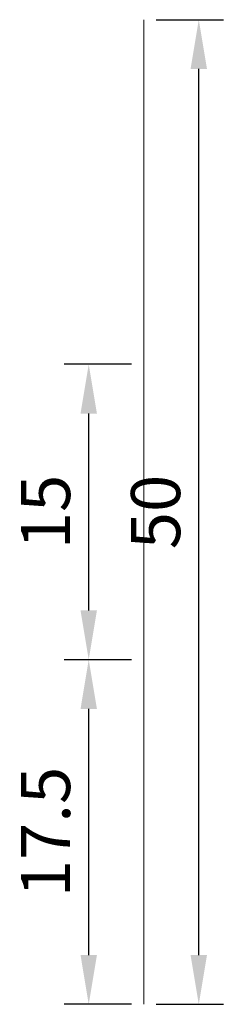
# Model space of a CAD drawing. Units: millimetres. Extents: x -6 to 912, y -42 to 105.
# Tile 1 of 2: x -6 to 4, y 55 to 105. Entities that reach past the tile are written whole.
import ezdxf

# ---------------------------------------------------------------- set-up
doc = ezdxf.new("R2010")
doc.units = ezdxf.units.MM
doc.layers.add('M-CONS', color=8, linetype='Continuous', lineweight=18)
doc.layers.add('M-DIMS', color=2, linetype='Continuous', lineweight=18)
doc.dimstyles.new('ISO-25', dxfattribs={"dimtxt": 2.5, "dimasz": 2.5, "dimexe": 1.25, "dimexo": 0.625, "dimtad": 1, "dimtxsty": 'Standard', "dimcen": 2.5, "dimadec": 0, "dimazin": 0, "dimtfac": 1, "dimtmove": 0, "dimatfit": 3, "dimfxl": 1, "dimarcsym": 0})

# ---------------------------------------------------------------- blocks, each defined once
blk = doc.blocks.new('*D8')
at = {"layer": 'Defpoints', "color": 0, "transparency": 16777216}
for p in [(0, 105.147), (2.8, 105.147), (0, 55.147)]:
    blk.add_point(p, dxfattribs=at)
at = {"layer": 'M-DIMS', "color": 0, "lineweight": -2, "transparency": 16777216}
for p, q in [((0.625, 105.147), (4.05, 105.147)), ((2.8, 57.647), (2.8, 102.647)), ((0.625, 55.147), (4.05, 55.147))]:
    blk.add_line(p, q, dxfattribs=at)
at = {"layer": 'M-DIMS', "color": 0, "transparency": 16777216}
for points in [[(2.383, 102.647), (3.217, 102.647), (2.8, 105.147)], [(2.383, 57.647), (3.217, 57.647), (2.8, 55.147)]]:
    blk.add_solid(points, dxfattribs=at)
at = {"layer": 'M-DIMS', "color": 0, "transparency": 16777216, "insert": (0.925, 80.147), "char_height": 2.5, "attachment_point": 5, "rotation": 90}
blk.add_mtext('50', dxfattribs=at)
blk = doc.blocks.new('*D9')
at = {"layer": 'Defpoints', "color": 0, "transparency": 16777216}
for p in [(-2.8, 72.647), (0, 72.647), (0, 55.147)]:
    blk.add_point(p, dxfattribs=at)
at = {"layer": 'M-DIMS', "color": 0, "lineweight": -2, "transparency": 16777216}
for p, q in [((-0.625, 72.647), (-4.05, 72.647)), ((-2.8, 57.647), (-2.8, 70.147)), ((-0.625, 55.147), (-4.05, 55.147))]:
    blk.add_line(p, q, dxfattribs=at)
at = {"layer": 'M-DIMS', "color": 0, "transparency": 16777216}
for points in [[(-3.217, 70.147), (-2.383, 70.147), (-2.8, 72.647)], [(-3.217, 57.647), (-2.383, 57.647), (-2.8, 55.147)]]:
    blk.add_solid(points, dxfattribs=at)
at = {"layer": 'M-DIMS', "color": 0, "transparency": 16777216, "insert": (-4.675, 63.897), "char_height": 2.5, "attachment_point": 5, "rotation": 90}
blk.add_mtext('17.5', dxfattribs=at)
blk = doc.blocks.new('*D10')
at = {"layer": 'Defpoints', "color": 0, "transparency": 16777216}
for p in [(-2.8, 87.647), (0, 87.647), (0, 72.647)]:
    blk.add_point(p, dxfattribs=at)
at = {"layer": 'M-DIMS', "color": 0, "lineweight": -2, "transparency": 16777216}
for p, q in [((-0.625, 87.647), (-4.05, 87.647)), ((-2.8, 75.147), (-2.8, 85.147)), ((-0.625, 72.647), (-4.05, 72.647))]:
    blk.add_line(p, q, dxfattribs=at)
at = {"layer": 'M-DIMS', "color": 0, "transparency": 16777216}
for points in [[(-3.217, 85.147), (-2.383, 85.147), (-2.8, 87.647)], [(-3.217, 75.147), (-2.383, 75.147), (-2.8, 72.647)]]:
    blk.add_solid(points, dxfattribs=at)
at = {"layer": 'M-DIMS', "color": 0, "transparency": 16777216, "insert": (-4.675, 80.147), "char_height": 2.5, "attachment_point": 5, "rotation": 90}
blk.add_mtext('15', dxfattribs=at)

msp = doc.modelspace()

# ---------------------------------------------------------------- linework, layer by layer
at = {"layer": 'M-CONS', "extrusion": (1, 0, 0)}
for p, q in [((0, 55.1469, 419.8255), (0, 105.1469, 419.8255)), ((0, 105.1469, 419.8255), (0, 105.1469, 459.8255)), ((0, 105.1469, 459.8255), (0, 87.6469, 459.8255)), ((0, 87.6469, 444.8255), (0, 87.6469, 459.8255)), ((0, 72.6469, 444.8255), (0, 72.6469, 459.8255)), ((0, 72.6469, 459.8255), (0, 55.1469, 459.8255)), ((0, 55.1469, 459.8255), (0, 55.1469, 419.8255))]:
    msp.add_line(p, q, dxfattribs=at)
msp.add_arc((80.1469, 444.8255), 7.5, 180, 0, dxfattribs=at)

# ---------------------------------------------------------------- dimensions: what is measured, and where the dimension line sits
at = {"layer": 'M-DIMS'}
for base, p1, p2, override, picture, middle in [((2.8, 105.1469), (0, 55.1469), (0, 105.1469), {"dimdec": 0, "dimlfac": 1, "dimrnd": 0, "dimzin": 0, "dimdsep": 46, "dimlunit": 2}, '*D8', (0.925, 80.1469)), ((-2.8, 87.6469), (0, 72.6469), (0, 87.6469), {"dimdec": 0, "dimlfac": 1, "dimrnd": 0, "dimzin": 0, "dimdsep": 46, "dimlunit": 2}, '*D10', (-4.675, 80.1469)), ((-2.8, 72.6469), (0, 55.1469), (0, 72.6469), {"dimdec": 1, "dimlfac": 1, "dimrnd": 0, "dimzin": 0, "dimdsep": 46, "dimlunit": 2}, '*D9', (-4.675, 63.8969))]:
    dim = msp.add_linear_dim(base=base, p1=p1, p2=p2, angle=90, dimstyle='ISO-25', override=override, dxfattribs=at)
    dim.commit()
    dim.dimension.update_dxf_attribs({"geometry": picture, "text_midpoint": middle})

doc.saveas('drawing.dxf')
